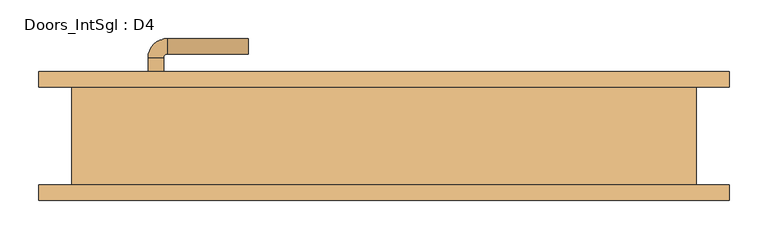
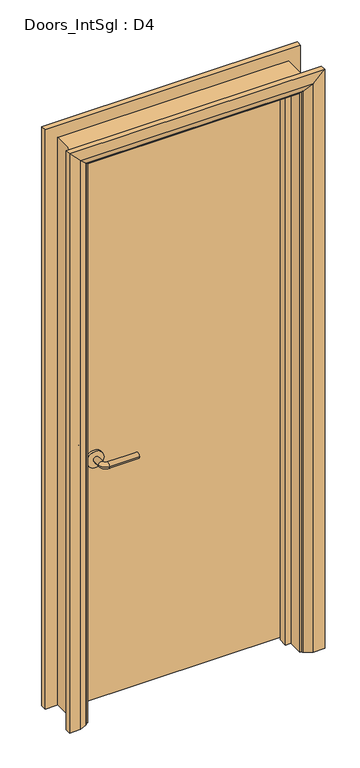
"""IFC4 building model written with IfcOpenShell, lengths in millimetres: door geometry, Doors_IntSgl : D4."""

from ifc_helpers import new_model, si_unit, point, frame, frame_2d, origin, place, context, project, spatial, polyline, circle_curve, ellipse_curve, trimmed, segment, composite_curve, outline, extrude, faceted_brep, source, transform, mapped, element, save
from ifc_brep_helpers import plane_surface, cylinder_surface, revolved_surface, advanced_brep


def doors_intsgl_d4_4271d8f6(model_context):
    return source(origin(), model_context, "Body", "SolidModel", [
        advanced_brep(
        [(-305.75, 17.5, 900.0), (-285.75, 17.5, 900.0), (-285.75, -12.5, 900.0), (-305.75, -12.5, 900.0), (-280.75, -17.5, 900.0), (-280.75, -37.5, 900.0), (-175.75, -37.5, 900.0), (-175.75, -17.5, 900.0)],
        [
            (0, 1, circle_curve(frame((-295.75, 17.5, 900.0), z_axis=(0.0, 1.0, 0.0), x_axis=(1.0, 0.0, 0.0)), 10.0)),
            (1, 0, circle_curve(frame((-295.75, 17.5, 900.0), z_axis=(0.0, 1.0, 0.0), x_axis=(1.0, 0.0, 0.0)), 10.0)),
            (1, 2),
            (2, 3, circle_curve(frame((-295.75, -12.5, 900.0), z_axis=(0.0, 1.0, 0.0), x_axis=(1.0, 0.0, 0.0)), 10.0)),
            (3, 0),
            (3, 2, circle_curve(frame((-295.75, -12.5, 900.0), z_axis=(0.0, 1.0, 0.0), x_axis=(1.0, 0.0, 0.0)), 10.0)),
            (4, 5, circle_curve(frame((-280.75, -27.5, 900.0), z_axis=(-1.0, 0.0, 0.0), x_axis=(0.0, 1.0, 0.0)), 10.0)),
            (5, 3, circle_curve(frame((-280.75, -12.5, 900.0), z_axis=(0.0, 0.0, -1.0), x_axis=(-1.0, 0.0, 0.0)), 25.0)),
            (2, 4, circle_curve(frame((-280.75, -12.5, 900.0), z_axis=(0.0, 0.0, 1.0), x_axis=(-1.0, 0.0, 0.0)), 5.0)),
            (5, 4, circle_curve(frame((-280.75, -27.5, 900.0), z_axis=(-1.0, 0.0, 0.0), x_axis=(0.0, 1.0, 0.0)), 10.0)),
            (6, 7, circle_curve(frame((-175.75, -27.5, 900.0), z_axis=(1.0, 0.0, 0.0), x_axis=(0.0, 1.0, 0.0)), 10.0)),
            (7, 6, circle_curve(frame((-175.75, -27.5, 900.0), z_axis=(1.0, 0.0, 0.0), x_axis=(0.0, 1.0, 0.0)), 10.0)),
            (4, 7),
            (6, 5),
        ],
        [
            plane_surface(frame((-295.75, 17.5, 900.0), z_axis=(0.0, 1.0, 0.0), x_axis=(0.0, 0.0, 1.0))),
            cylinder_surface(frame((-295.75, 17.5, 900.0), z_axis=(0.0, 1.0, 0.0), x_axis=(1.0, 0.0, 0.0)), 10.0),
            revolved_surface(trimmed(ellipse_curve(frame((-295.75, -12.5, 900.0), z_axis=(0.0, -1.0, 0.0), x_axis=(1.0, 0.0, 0.0)), 10.0, 10.0), [point((-305.75, -12.5, 900.0))], [point((-285.75, -12.5, 900.0))], True, "CARTESIAN"), (-280.75, -12.5, 900.0), (0.0, 0.0, -1.0)),
            revolved_surface(trimmed(ellipse_curve(frame((-295.75, -12.5, 900.0), z_axis=(0.0, -1.0, 0.0), x_axis=(1.0, 0.0, 0.0)), 10.0, 10.0), [point((-285.75, -12.5, 900.0))], [point((-305.75, -12.5, 900.0))], True, "CARTESIAN"), (-280.75, -12.5, 900.0), (0.0, 0.0, -1.0)),
            plane_surface(frame((-175.75, -27.5, 900.0), z_axis=(1.0, 0.0, 0.0), x_axis=(0.0, 0.0, 1.0))),
            cylinder_surface(frame((-280.75, -27.5, 900.0), z_axis=(-1.0, 0.0, 0.0), x_axis=(0.0, 1.0, 0.0)), 10.0),
        ],
        [
            (0, [[1, 2]]),
            (1, [[3, 4, 5, -2]]),
            (1, [[-5, 6, -3, -1]]),
            (2, [[7, 8, -4, 9]]),
            (3, [[10, -9, -6, -8]]),
            (4, [[11, 12]]),
            (5, [[13, -11, 14, -7]]),
            (5, [[-14, -12, -13, -10]]),
        ],
    ),
        extrude(outline(composite_curve([segment(trimmed(circle_curve(frame_2d((900.0, -298.25)), 30.0), [point((900.0, -328.25))], [point((900.0, -268.25))], False, "CARTESIAN"), True, "CONTINUOUS"), segment(trimmed(circle_curve(frame_2d((900.0, -298.25)), 30.0), [point((900.0, -268.25))], [point((900.0, -328.25))], False, "CARTESIAN"), True, "CONTINUOUS")], self_intersect=False)), frame((0.0, 17.5, 0.0), z_axis=(0.0, 1.0, 0.0), x_axis=(0.0, 0.0, 1.0)), (0.0, 0.0, 1.0), 8.0),
        advanced_brep(
        [(-305.75, 71.5, 900.0), (-285.75, 71.5, 900.0), (-305.75, 101.5, 900.0), (-285.75, 101.5, 900.0), (-280.75, 106.5, 900.0), (-280.75, 126.5, 900.0), (-175.75, 126.5, 900.0), (-175.75, 106.5, 900.0)],
        [
            (0, 1, circle_curve(frame((-295.75, 71.5, 900.0), z_axis=(0.0, -1.0, 0.0), x_axis=(1.0, 0.0, 0.0)), 10.0)),
            (1, 0, circle_curve(frame((-295.75, 71.5, 900.0), z_axis=(0.0, -1.0, 0.0), x_axis=(1.0, 0.0, 0.0)), 10.0)),
            (0, 2),
            (2, 3, circle_curve(frame((-295.75, 101.5, 900.0), z_axis=(0.0, -1.0, 0.0), x_axis=(1.0, 0.0, 0.0)), 10.0)),
            (3, 1),
            (3, 2, circle_curve(frame((-295.75, 101.5, 900.0), z_axis=(0.0, -1.0, 0.0), x_axis=(1.0, 0.0, 0.0)), 10.0)),
            (4, 3, circle_curve(frame((-280.75, 101.5, 900.0), z_axis=(0.0, 0.0, 1.0), x_axis=(-1.0, 0.0, 0.0)), 5.0)),
            (2, 5, circle_curve(frame((-280.75, 101.5, 900.0), z_axis=(0.0, 0.0, -1.0), x_axis=(-1.0, 0.0, 0.0)), 25.0)),
            (5, 4, circle_curve(frame((-280.75, 116.5, 900.0), z_axis=(-1.0, 0.0, 0.0), x_axis=(0.0, -1.0, 0.0)), 10.0)),
            (4, 5, circle_curve(frame((-280.75, 116.5, 900.0), z_axis=(-1.0, 0.0, 0.0), x_axis=(0.0, -1.0, 0.0)), 10.0)),
            (6, 7, circle_curve(frame((-175.75, 116.5, 900.0), z_axis=(1.0, 0.0, 0.0), x_axis=(0.0, -1.0, 0.0)), 10.0)),
            (7, 6, circle_curve(frame((-175.75, 116.5, 900.0), z_axis=(1.0, 0.0, 0.0), x_axis=(0.0, -1.0, 0.0)), 10.0)),
            (5, 6),
            (7, 4),
        ],
        [
            plane_surface(frame((-295.75, 71.5, 900.0), z_axis=(0.0, -1.0, 0.0), x_axis=(0.0, 0.0, 1.0))),
            cylinder_surface(frame((-295.75, 71.5, 900.0), z_axis=(0.0, -1.0, 0.0), x_axis=(1.0, 0.0, 0.0)), 10.0),
            revolved_surface(trimmed(ellipse_curve(frame((-295.75, 101.5, 900.0), z_axis=(0.0, -1.0, 0.0), x_axis=(1.0, 0.0, 0.0)), 10.0, 10.0), [point((-305.75, 101.5, 900.0))], [point((-285.75, 101.5, 900.0))], True, "CARTESIAN"), (-280.75, 101.5, 900.0), (0.0, 0.0, -1.0)),
            revolved_surface(trimmed(ellipse_curve(frame((-295.75, 101.5, 900.0), z_axis=(0.0, -1.0, 0.0), x_axis=(1.0, 0.0, 0.0)), 10.0, 10.0), [point((-285.75, 101.5, 900.0))], [point((-305.75, 101.5, 900.0))], True, "CARTESIAN"), (-280.75, 101.5, 900.0), (0.0, 0.0, -1.0)),
            plane_surface(frame((-175.75, 116.5, 900.0), z_axis=(1.0, 0.0, 0.0), x_axis=(0.0, 0.0, 1.0))),
            cylinder_surface(frame((-280.75, 116.5, 900.0), z_axis=(-1.0, 0.0, 0.0), x_axis=(0.0, -1.0, 0.0)), 10.0),
        ],
        [
            (0, [[1, 2]]),
            (1, [[-1, 3, 4, 5]]),
            (1, [[-2, -5, 6, -3]]),
            (2, [[7, -4, 8, 9]]),
            (3, [[-8, -6, -7, 10]]),
            (4, [[11, 12]]),
            (5, [[-9, 13, -12, 14]]),
            (5, [[-10, -14, -11, -13]]),
        ],
    ),
        extrude(outline(composite_curve([segment(trimmed(circle_curve(frame_2d((900.0, -298.25)), 30.0), [point((900.0, -328.25))], [point((900.0, -268.25))], False, "CARTESIAN"), True, "CONTINUOUS"), segment(trimmed(circle_curve(frame_2d((900.0, -298.25)), 30.0), [point((900.0, -268.25))], [point((900.0, -328.25))], False, "CARTESIAN"), True, "CONTINUOUS")], self_intersect=False)), frame((0.0, 63.5, 0.0), z_axis=(0.0, 1.0, 0.0), x_axis=(0.0, 0.0, 1.0)), (0.0, 0.0, 1.0), 8.0),
        extrude(outline(polyline([(370.75, 25.5), (-370.75, 25.5), (-370.75, 63.5), (370.75, 63.5), (370.75, 25.5)])), frame((0.0, 0.0, 8.0), z_axis=(0.0, 0.0, 1.0), x_axis=(1.0, 0.0, 0.0)), (0.0, 0.0, 1.0), 2060.0),
        advanced_brep(
        [(447.75, 83.5, 0.0), (447.75, 63.5, 0.0), (377.75, 63.5, 0.0), (381.75, 69.5, 0.0), (407.75, 83.5, 0.0), (447.75, 83.5, 2145.0), (447.75, 63.5, 2145.0), (-447.75, 63.5, 2145.0), (-447.75, 63.5, 0.0), (-377.75, 63.5, 0.0), (-377.75, 63.5, 2075.0), (377.75, 63.5, 2075.0), (381.75, 69.5, 2079.0), (407.75, 83.5, 2105.0), (-407.75, 83.5, 2105.0), (-407.75, 83.5, 0.0), (-447.75, 83.5, 0.0), (-447.75, 83.5, 2145.0), (-381.75, 69.5, 0.0), (-381.75, 69.5, 2079.0)],
        [
            (0, 1),
            (1, 2),
            (2, 3, circle_curve(frame((385.75, 62.5, 0.0), z_axis=(0.0, 0.0, -1.0), x_axis=(1.0, 0.0, 0.0)), 8.0622577)),
            (3, 4),
            (4, 0),
            (0, 5),
            (5, 6),
            (6, 1),
            (6, 7),
            (7, 8),
            (8, 9),
            (9, 10),
            (10, 11),
            (11, 2),
            (11, 12, ellipse_curve(frame((385.75, 62.5, 2083.0), z_axis=(0.7071067811865475, 0.0, -0.7071067811865475), x_axis=(-0.7071067811865474, 0.0, -0.7071067811865476)), 11.4017543, 8.0622577)),
            (12, 3),
            (12, 13),
            (13, 4),
            (13, 14),
            (14, 15),
            (15, 16),
            (16, 17),
            (17, 5),
            (7, 17),
            (16, 8),
            (15, 18),
            (18, 9, circle_curve(frame((-385.75, 62.5, 0.0), z_axis=(0.0, 0.0, -1.0), x_axis=(-1.0, 0.0, 0.0)), 8.0622577)),
            (19, 10, ellipse_curve(frame((-385.75, 62.5, 2083.0), z_axis=(-0.7071067811865475, 0.0, -0.7071067811865475), x_axis=(-0.7071067811865474, 0.0, 0.7071067811865476)), 11.4017543, 8.0622577)),
            (18, 19),
            (14, 19),
            (19, 12),
        ],
        [
            plane_surface(frame((377.75, 63.5, 0.0), z_axis=(0.0, 0.0, -1.0), x_axis=(0.0, -1.0, 0.0))),
            plane_surface(frame((447.75, 83.5, 0.0), z_axis=(1.0, 0.0, 0.0), x_axis=(0.0, 0.0, 1.0))),
            plane_surface(frame((447.75, 63.5, 0.0), z_axis=(0.0, -1.0, 0.0), x_axis=(0.0, 0.0, 1.0))),
            cylinder_surface(frame((385.75, 62.5, 0.0), z_axis=(0.0, 0.0, -1.0), x_axis=(1.0, 0.0, 0.0)), 8.0622577),
            plane_surface(frame((381.75, 69.5, 0.0), z_axis=(-0.4740998230350126, 0.880471099922178, 0.0), x_axis=(0.0, 0.0, 1.0))),
            plane_surface(frame((407.75, 83.5, 0.0), z_axis=(0.0, 1.0, 0.0), x_axis=(0.0, 0.0, 1.0))),
            plane_surface(frame((-447.75, 83.5, 2145.0), z_axis=(-1.0, 0.0, 0.0), x_axis=(0.0, 0.0, -1.0))),
            plane_surface(frame((-377.75, 63.5, 0.0), z_axis=(0.0, 0.0, -1.0), x_axis=(0.0, -1.0, 0.0))),
            cylinder_surface(frame((-385.75, 62.5, 2075.0), z_axis=(0.0, 0.0, 1.0), x_axis=(-1.0, 0.0, 0.0)), 8.0622577),
            plane_surface(frame((-381.75, 69.5, 2079.0), z_axis=(0.47409982303501824, 0.8804710999221749, 0.0), x_axis=(0.0, 0.0, -1.0))),
            plane_surface(frame((447.75, 83.5, 2145.0), z_axis=(0.0, 0.0, 1.0), x_axis=(-1.0, 0.0, 0.0))),
            cylinder_surface(frame((377.75, 62.5, 2083.0), z_axis=(1.0, 0.0, 0.0), x_axis=(0.0, 0.0, 1.0)), 8.0622577),
            plane_surface(frame((381.75, 69.5, 2079.0), z_axis=(0.0, 0.8804710999221764, -0.4740998230350154), x_axis=(-1.0, 0.0, 0.0))),
        ],
        [
            (0, [[1, 2, 3, 4, 5]]),
            (1, [[-1, 6, 7, 8]]),
            (2, [[-2, -8, 9, 10, 11, 12, 13, 14]]),
            (3, [[-3, -14, 15, 16]]),
            (4, [[-4, -16, 17, 18]]),
            (5, [[-5, -18, 19, 20, 21, 22, 23, -6]]),
            (6, [[24, -22, 25, -10]]),
            (7, [[-21, 26, 27, -11, -25]]),
            (8, [[28, -12, -27, 29]]),
            (9, [[30, -29, -26, -20]]),
            (10, [[-7, -23, -24, -9]]),
            (11, [[-15, -13, -28, 31]]),
            (12, [[-17, -31, -30, -19]]),
        ],
    ),
        extrude(outline(polyline([(0.0, -372.75), (0.0, -353.75), (2051.0, -353.75), (2051.0, 353.75), (0.0, 353.75), (0.0, 372.75), (2070.0, 372.75), (2070.0, -372.75), (0.0, -372.75)])), frame((0.0, -8.5, 0.0), z_axis=(0.0, 1.0, 0.0), x_axis=(0.0, 0.0, 1.0)), (0.0, 0.0, 1.0), 32.0),
        advanced_brep(
        [(-447.75, -83.5, 0.0), (-447.75, -63.5, 0.0), (-377.75, -63.5, 0.0), (-381.75, -69.5, 0.0), (-407.75, -83.5, 0.0), (-447.75, -83.5, 2145.0), (-447.75, -63.5, 2145.0), (-377.75, -63.5, 2075.0), (-381.75, -69.5, 2079.0), (-407.75, -83.5, 2105.0), (447.75, -83.5, 0.0), (407.75, -83.5, 0.0), (381.75, -69.5, 0.0), (377.75, -63.5, 0.0), (447.75, -63.5, 0.0), (447.75, -83.5, 2145.0), (407.75, -83.5, 2105.0), (381.75, -69.5, 2079.0), (377.75, -63.5, 2075.0), (447.75, -63.5, 2145.0)],
        [
            (0, 1),
            (1, 2),
            (2, 3, circle_curve(frame((-385.75, -62.5, 0.0), z_axis=(0.0, 0.0, -1.0), x_axis=(-1.0, 0.0, 0.0)), 8.0622577)),
            (3, 4),
            (4, 0),
            (0, 5),
            (5, 6),
            (6, 1),
            (6, 7),
            (7, 2),
            (7, 8, ellipse_curve(frame((-385.75, -62.5, 2083.0), z_axis=(-0.7071067811865475, 0.0, -0.7071067811865475), x_axis=(0.7071067811865474, 0.0, -0.7071067811865476)), 11.4017543, 8.0622577)),
            (8, 3),
            (8, 9),
            (9, 4),
            (9, 5),
            (10, 11),
            (11, 12),
            (12, 13, circle_curve(frame((385.75, -62.5, 0.0), z_axis=(0.0, 0.0, -1.0), x_axis=(1.0, 0.0, 0.0)), 8.0622577)),
            (13, 14),
            (14, 10),
            (15, 16),
            (16, 11),
            (10, 15),
            (16, 17),
            (17, 12),
            (17, 18, ellipse_curve(frame((385.75, -62.5, 2083.0), z_axis=(0.7071067811865475, 0.0, -0.7071067811865475), x_axis=(0.7071067811865474, 0.0, 0.7071067811865476)), 11.4017543, 8.0622577)),
            (18, 13),
            (18, 19),
            (19, 14),
            (19, 15),
            (5, 15),
            (19, 6),
            (18, 7),
            (17, 8),
            (16, 9),
        ],
        [
            plane_surface(frame((-377.75, -136.3010989, 0.0), z_axis=(0.0, 0.0, -1.0), x_axis=(1.0, 0.0, 0.0))),
            plane_surface(frame((-447.75, -83.5, 0.0), z_axis=(-1.0, 0.0, 0.0), x_axis=(0.0, 0.0, 1.0))),
            plane_surface(frame((-447.75, -63.5, 0.0), z_axis=(0.0, 1.0, 0.0), x_axis=(0.0, 0.0, 1.0))),
            cylinder_surface(frame((-385.75, -62.5, 0.0), z_axis=(0.0, 0.0, -1.0), x_axis=(-1.0, 0.0, 0.0)), 8.0622577),
            plane_surface(frame((-381.75, -69.5, 0.0), z_axis=(0.4740998230350183, -0.8804710999221749, 0.0), x_axis=(0.0, 0.0, 1.0))),
            plane_surface(frame((-407.75, -83.5, 0.0), z_axis=(0.0, -1.0, 0.0), x_axis=(0.0, 0.0, 1.0))),
            plane_surface(frame((377.75, -136.3010989, 0.0), z_axis=(0.0, 0.0, -1.0), x_axis=(-1.0, 0.0, 0.0))),
            plane_surface(frame((407.75, -83.5, 2105.0), z_axis=(0.0, -1.0, 0.0), x_axis=(0.0, 0.0, -1.0))),
            plane_surface(frame((381.75, -69.5, 2079.0), z_axis=(-0.4740998230350183, -0.8804710999221749, 0.0), x_axis=(0.0, 0.0, -1.0))),
            cylinder_surface(frame((385.75, -62.5, 2075.0), z_axis=(0.0, 0.0, 1.0), x_axis=(1.0, 0.0, 0.0)), 8.0622577),
            plane_surface(frame((447.75, -63.5, 2145.0), z_axis=(0.0, 1.0, 0.0), x_axis=(0.0, 0.0, -1.0))),
            plane_surface(frame((447.75, -83.5, 2145.0), z_axis=(1.0, 0.0, 0.0), x_axis=(0.0, 0.0, -1.0))),
            plane_surface(frame((-447.75, -83.5, 2145.0), z_axis=(0.0, 0.0, 1.0), x_axis=(1.0, 0.0, 0.0))),
            plane_surface(frame((-447.75, -63.5, 2145.0), z_axis=(0.0, 1.0, 0.0), x_axis=(1.0, 0.0, 0.0))),
            cylinder_surface(frame((-377.75, -62.5, 2083.0), z_axis=(-1.0, 0.0, 0.0), x_axis=(0.0, 0.0, 1.0)), 8.0622577),
            plane_surface(frame((-381.75, -69.5, 2079.0), z_axis=(0.0, -0.8804710999221749, -0.4740998230350183), x_axis=(1.0, 0.0, 0.0))),
            plane_surface(frame((-407.75, -83.5, 2105.0), z_axis=(0.0, -1.0, 0.0), x_axis=(1.0, 0.0, 0.0))),
        ],
        [
            (0, [[1, 2, 3, 4, 5]]),
            (1, [[-1, 6, 7, 8]]),
            (2, [[-2, -8, 9, 10]]),
            (3, [[-3, -10, 11, 12]]),
            (4, [[-4, -12, 13, 14]]),
            (5, [[-5, -14, 15, -6]]),
            (6, [[16, 17, 18, 19, 20]]),
            (7, [[21, 22, -16, 23]]),
            (8, [[24, 25, -17, -22]]),
            (9, [[26, 27, -18, -25]]),
            (10, [[28, 29, -19, -27]]),
            (11, [[30, -23, -20, -29]]),
            (12, [[-7, 31, -30, 32]]),
            (13, [[-9, -32, -28, 33]]),
            (14, [[-11, -33, -26, 34]]),
            (15, [[-13, -34, -24, 35]]),
            (16, [[-15, -35, -21, -31]]),
        ],
    ),
        faceted_brep([(-372.75, 63.5, 0.0), (-372.75, -63.5, 0.0), (-404.75, -63.5, 0.0), (-404.75, 63.5, 0.0), (-372.75, 63.5, 2070.0), (-372.75, -63.5, 2070.0), (-404.75, -63.5, 2102.0), (-404.75, 63.5, 2102.0), (372.75, 63.5, 0.0), (404.75, 63.5, 0.0), (404.75, -63.5, 0.0), (372.75, -63.5, 0.0), (372.75, 63.5, 2070.0), (404.75, 63.5, 2102.0), (404.75, -63.5, 2102.0), (372.75, -63.5, 2070.0)], [[[0, 1, 2, 3]], [[1, 0, 4, 5]], [[2, 1, 5, 6]], [[3, 2, 6, 7]], [[0, 3, 7, 4]], [[8, 9, 10, 11]], [[12, 13, 9, 8]], [[13, 14, 10, 9]], [[14, 15, 11, 10]], [[15, 12, 8, 11]], [[5, 4, 12, 15]], [[6, 5, 15, 14]], [[7, 6, 14, 13]], [[4, 7, 13, 12]]]),
    ])


if __name__ == "__main__":
    model = new_model("IFC4")
    model_context = context("Model", 3, world=origin())
    ifc_project = project(units=[si_unit("LENGTHUNIT", "METRE", prefix="MILLI")], contexts=[model_context])
    site = spatial("IfcSite", under=ifc_project)
    building = spatial("IfcBuilding", under=site)
    placement = place(None, origin())
    doors_intsgl_d4_shape = doors_intsgl_d4_4271d8f6(model_context)
    element("IfcDoor", 1, ObjectType="Doors_IntSgl : D4", at=placement, inside=building, context=model_context, shape_type="MappedRepresentation", body=[
        mapped(doors_intsgl_d4_shape, transform((0.0, 0.0, 0.0), x_axis=(1.0, 0.0, 0.0), y_axis=(0.0, 1.0, 0.0), z_axis=(0.0, 0.0, 1.0))),
    ])
    save(model, "model.ifc")

# Revit data of these elements
# Type "Doors_IntSgl : D4"
#   Type Mark = "50"
#   Type Comments = "Internal Single"
#   Operation = "SingleSwingRight"
#   Manufacturer = "Revit"
#   Keynote = "L20"
#   Description = "Internal Single Door"
#   Analytic Construction = "Metal"
#   UnderCut = 0' - 0.31496"
#   Tolerance = 0' - 0.07874"
#   Thickness = 0' - 1.49606"
#   Thermal Resistance (R) = 0.270117 (m²·K)/W
#   Structural Tolerance = 0' - 0.31496"
#   StopDepth = 0' - 1.25984"
#   Stop Thickness = 0' - 0.74803"
#   Rough Width = 2' - 8 1/2"
#   Rough Height = 6' - 11.07087"
#   Height to Top Lock Rail = 3' - 3.37008"
#   Heat Transfer Coefficient (U) = 3.7021 W/(m²·K)
#   Handle Z Distance = 2' - 11.43307"
#   Handle X Distance = 0' - 2.95276"
#   Frame Thickness = 0' - 1.25984"
#   Door Panel Width = 2' - 5.19291"
#   Door Panel Thickness = 0' - 1.49606"
#   Door Panel Offset = 0' - 0"
#   Height = 6' - 11.07087"
#   Width = 2' - 8 1/2"
#   Door Panel Height = 6' - 9.10236"
#   Architrave Setback = 0' - 0.19685"
#   Vis - Ironmongery = yes
#   Material Ironmongery = Door - Handle
#   Material Frame = Door - Frame/Mullion (1)
#   Material Door = Door - Panel
#   Material Architrave = Door - Architrave
#   Visual Light Transmittance = 0
#   Solar Heat Gain Coefficient = 0
#   Function = (empty or 0)
#   Wall Closure = (empty or 0)
# Element 1 (IfcDoor, "Doors_IntSgl : D4")
#   Materials on its faces: "Door - Architrave", "Door - Handle", "Door - Frame/Mullion (1)", "Door - Panel"
# Materials
#   "Door - Handle": colour RGB 0 0 0, transparency 0, Keynote = "P21", Cost = 0
#   "Door - Frame/Mullion (1)": class "Wood", colour RGB 212 179 113, transparency 0, Keynote = "L20", Cost = 0
#   "Door - Panel": class "Wood", colour RGB 210 159 95, transparency 0, Keynote = "L20", Cost = 0
#   "Door - Architrave": class "Wood", colour RGB 154 90 5, transparency 0, Keynote = "P20", Cost = 0
